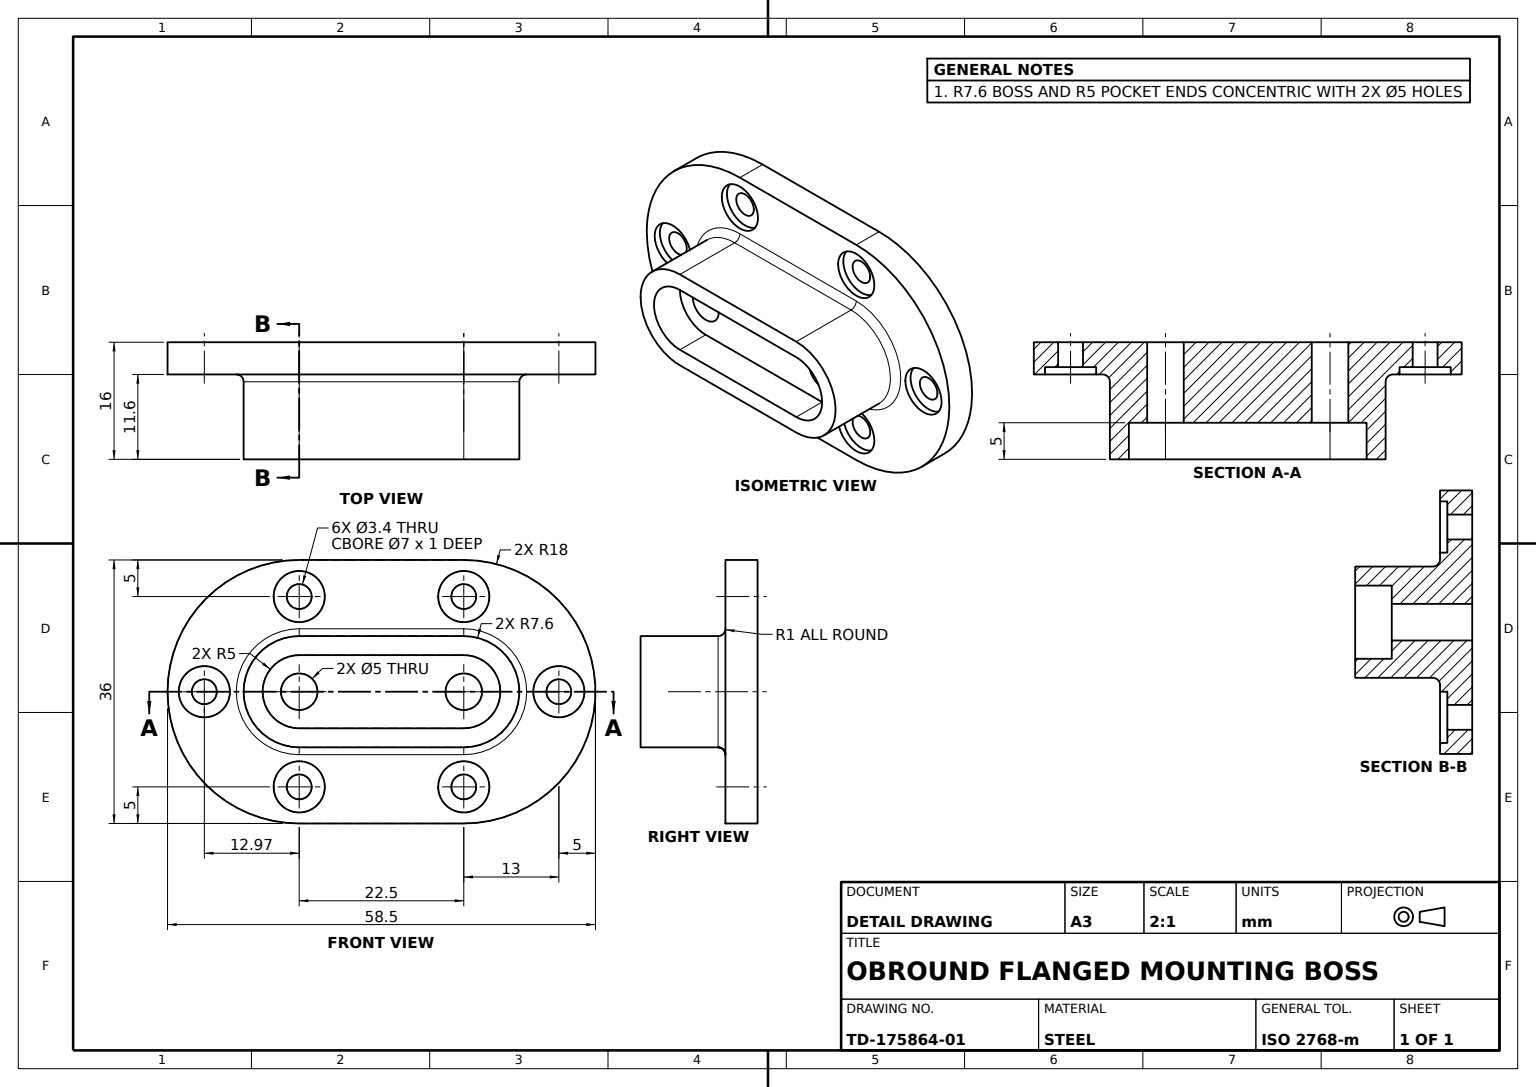
from build123d import *

# Parameters (mm, degrees)
OVAL_BASE_FLANGE_DEPTH       = 4.4
RAISED_OBROUND_HOUSING_DEPTH = 11.6
HOUSING_SLOT_R5_DEPTH        = 5
MOUNTING_HOLES_SKETCH_R      = 1.7
MOUNTING_HOLES_6X_3_4_DEPTH  = 5
COUNTERBORE_SKETCH_R         = 3.5
COUNTERBORES_6X_7_DEPTH      = 1
SLOT_THROUGH_CUT_SKETCH_R    = 2.5
SLOT_THROUGH_CUT_DEPTH       = 37.063312383
HOUSING_BASE_FILLET_R1_R     = 1


with BuildPart() as part:
    # Flange Profile Sketch → Oval Base Flange (new body)
    with BuildSketch(Plane.XY):
        with BuildLine():
            Line((-11.25, 18), (11.25, 18))
            ThreePointArc((11.25, 18), (29.25, 0), (11.25, -18))
            Line((11.25, -18), (-11.25, -18))
            ThreePointArc((-11.25, -18), (-29.25, 0), (-11.25, 18))
        make_face()
    extrude(amount=OVAL_BASE_FLANGE_DEPTH)

    # Housing Profile Sketch → Raised Obround Housing (add)
    with BuildSketch(Plane.XY.offset(4.4)):
        with BuildLine():
            Line((-11.25, 7.6), (11.25, 7.6))
            ThreePointArc((11.25, 7.6), (18.85, 0), (11.25, -7.6))
            Line((11.25, -7.6), (-11.25, -7.6))
            ThreePointArc((-11.25, -7.6), (-18.85, 0), (-11.25, 7.6))
        make_face()
    extrude(amount=RAISED_OBROUND_HOUSING_DEPTH)

    # Housing Slot Sketch → Housing Slot R5 (cut)
    with BuildSketch(Plane.XY.offset(16)):
        with BuildLine():
            Line((-11.25, 5), (11.25, 5))
            ThreePointArc((11.25, 5), (16.25, 0), (11.25, -5))
            Line((11.25, -5), (-11.25, -5))
            ThreePointArc((-11.25, -5), (-16.25, 0), (-11.25, 5))
        make_face()
    extrude(amount=-HOUSING_SLOT_R5_DEPTH, mode=Mode.SUBTRACT)

    # Mounting Holes Sketch → Mounting Holes 6xØ3.4 (cut)
    with BuildSketch(Plane.XY.offset(4.4)):
        with Locations((-24.22204296, 0)):
            Circle(MOUNTING_HOLES_SKETCH_R)
        with Locations((-11.25, 13)):
            Circle(MOUNTING_HOLES_SKETCH_R)
        with Locations((11.25, 13)):
            Circle(MOUNTING_HOLES_SKETCH_R)
        with Locations((24.25, 0)):
            Circle(MOUNTING_HOLES_SKETCH_R)
        with Locations((11.25, -13)):
            Circle(MOUNTING_HOLES_SKETCH_R)
        with Locations((-11.25, -13)):
            Circle(MOUNTING_HOLES_SKETCH_R)
    extrude(amount=-MOUNTING_HOLES_6X_3_4_DEPTH, mode=Mode.SUBTRACT)

    # Counterbore Sketch → Counterbores 6xØ7 (cut)
    with BuildSketch(Plane.XY.offset(4.4)):
        with Locations((-24.22204296, 0)):
            Circle(COUNTERBORE_SKETCH_R)
        with Locations((-11.25, 13)):
            Circle(COUNTERBORE_SKETCH_R)
        with Locations((11.25, 13)):
            Circle(COUNTERBORE_SKETCH_R)
        with Locations((24.25, 0)):
            Circle(COUNTERBORE_SKETCH_R)
        with Locations((11.25, -13)):
            Circle(COUNTERBORE_SKETCH_R)
        with Locations((-11.25, -13)):
            Circle(COUNTERBORE_SKETCH_R)
    extrude(amount=-COUNTERBORES_6X_7_DEPTH, mode=Mode.SUBTRACT)

    # Slot Through Cut Sketch → Slot Through Cut (cut, through all)
    with BuildSketch(Plane.XY.offset(11)):
        with Locations((-11.25, 0)):
            Circle(SLOT_THROUGH_CUT_SKETCH_R)
        with Locations((11.25, 0)):
            Circle(SLOT_THROUGH_CUT_SKETCH_R)
    extrude(amount=-SLOT_THROUGH_CUT_DEPTH, mode=Mode.SUBTRACT)

    # Housing Base Fillet R1
    housing_base_fillet_r1_edges = [part.edges().sort_by_distance(p)[0] for p in [
        (-18.85, 0, 4.4),
        (0, -7.6, 4.4),
        (18.85, 0, 4.4),
        (0, 7.6, 4.4),
    ]]
    fillet(housing_base_fillet_r1_edges, radius=HOUSING_BASE_FILLET_R1_R)


solid = part.part
